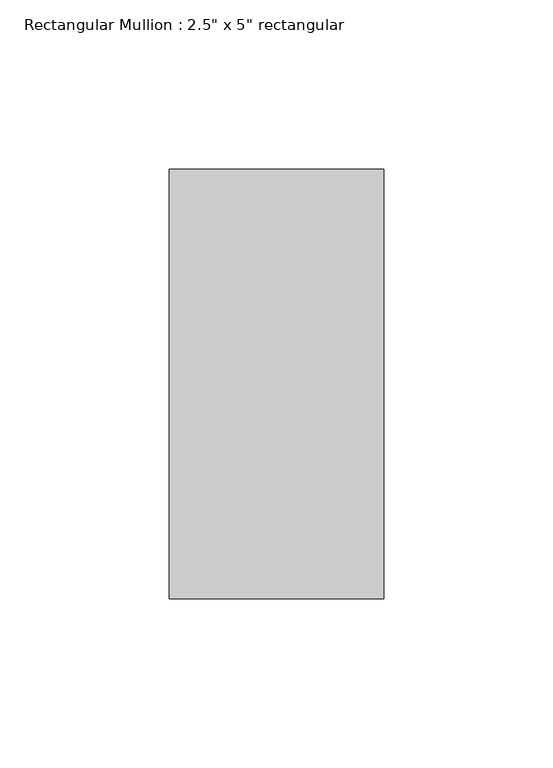
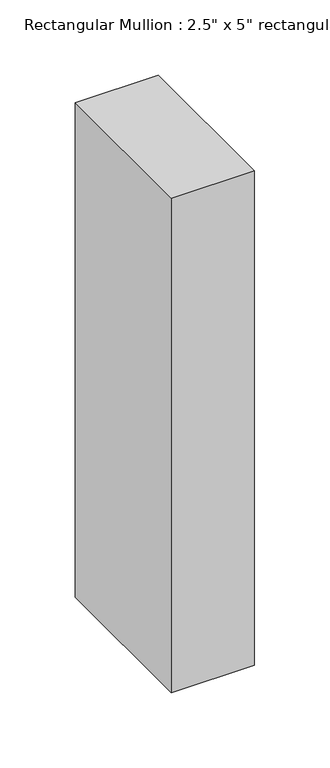
"""IFC4 building model written with IfcOpenShell, lengths in millimetres: member geometry."""

from ifc_helpers import new_model, si_unit, frame, origin, place, context, project, spatial, polyline, outline, extrude, source, transform, mapped, element, save


def member_1ad5418d(model_context):
    return source(origin(), model_context, "Body", "SweptSolid", [
        extrude(outline(polyline([(0.0, 63.5), (0.0, -63.5), (-63.5, -63.5), (-63.5, 63.5), (0.0, 63.5)])), frame((0.0, 0.0, -400.05), z_axis=(0.0, 0.0, 1.0), x_axis=(1.0, 0.0, 0.0)), (0.0, 0.0, 1.0), 400.05),
    ])


if __name__ == "__main__":
    model = new_model("IFC4")
    model_context = context("Model", 3, world=origin())
    ifc_project = project(units=[si_unit("LENGTHUNIT", "METRE", prefix="MILLI")], contexts=[model_context])
    site = spatial("IfcSite", under=ifc_project)
    building = spatial("IfcBuilding", under=site)
    placement = place(None, origin())
    member_shape = member_1ad5418d(model_context)
    element("IfcMember", 1, ObjectType="Rectangular Mullion : 2.5\" x 5\" rectangular", at=placement, inside=building, context=model_context, shape_type="MappedRepresentation", body=[
        mapped(member_shape, transform((0.0, 0.0, 0.0), x_axis=(1.0, 0.0, 0.0), y_axis=(0.0, 1.0, 0.0), z_axis=(0.0, 0.0, 1.0))),
    ])
    save(model, "model.ifc")

# Revit data of these elements
# Type "Rectangular Mullion : 2.5\" x 5\" rectangular"
#   built-in parameter 1007304 = 0.416667 (stored number, unit not read)
#   built-in parameter 1007301 = 0.104167 (stored number, unit not read)
#   built-in parameter 1007300 = 0.104167 (stored number, unit not read)
# Element 1 (IfcMember, "Rectangular Mullion : 2.5\" x 5\" rectangular")
#   Materials on its faces: "Aluminum"
# Materials
#   "Aluminum": class "Metal", colour RGB 247 247 247, transparency 0, Description = "Aluminum 6061", Cost = 0
